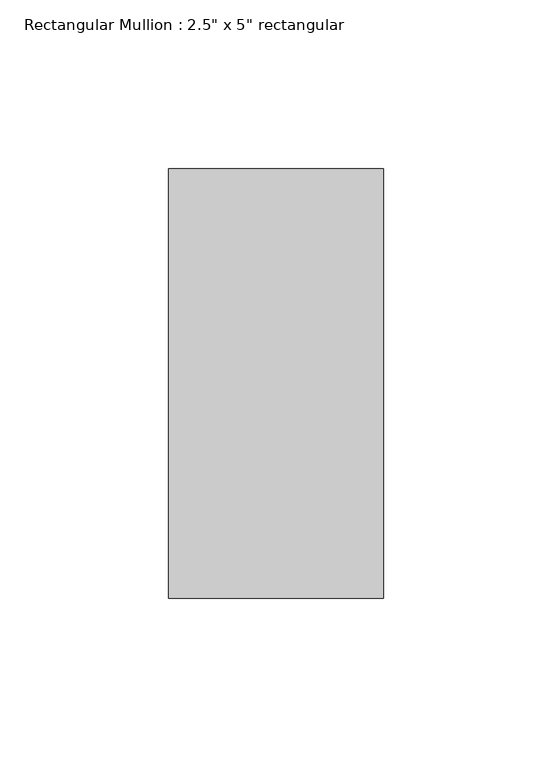
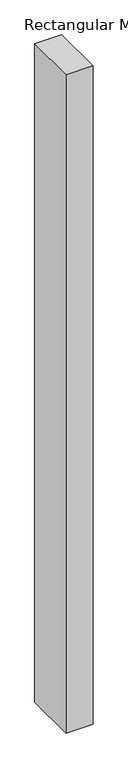
"""IFC4 building model written with IfcOpenShell, lengths in millimetres: member geometry."""

from ifc_helpers import new_model, si_unit, frame, origin, place, context, project, spatial, polyline, outline, extrude, source, transform, mapped, element, save


def member_e2524bce(model_context):
    return source(origin(), model_context, "Body", "SweptSolid", [
        extrude(outline(polyline([(0.0, 63.5), (0.0, -63.5), (-63.5, -63.5), (-63.5, 63.5), (0.0, 63.5)])), frame((0.0, 0.0, -1634.3549218), z_axis=(0.0, 0.0, 1.0), x_axis=(1.0, 0.0, 0.0)), (0.0, 0.0, 1.0), 1634.3549218),
    ])


if __name__ == "__main__":
    model = new_model("IFC4")
    model_context = context("Model", 3, world=origin())
    ifc_project = project(units=[si_unit("LENGTHUNIT", "METRE", prefix="MILLI")], contexts=[model_context])
    site = spatial("IfcSite", under=ifc_project)
    building = spatial("IfcBuilding", under=site)
    placement = place(None, origin())
    member_shape = member_e2524bce(model_context)
    element("IfcMember", 1, ObjectType="Rectangular Mullion : 2.5\" x 5\" rectangular", at=placement, inside=building, context=model_context, shape_type="MappedRepresentation", body=[
        mapped(member_shape, transform((0.0, 0.0, 0.0), x_axis=(1.0, 0.0, 0.0), y_axis=(0.0, 1.0, 0.0), z_axis=(0.0, 0.0, 1.0))),
    ])
    save(model, "model.ifc")

# Revit data of these elements
# Type "Rectangular Mullion : 2.5\" x 5\" rectangular"
#   built-in parameter 1007304 = 0.416667 (stored number, unit not read)
#   built-in parameter 1007301 = 0.104167 (stored number, unit not read)
#   built-in parameter 1007300 = 0.104167 (stored number, unit not read)
# Element 1 (IfcMember, "Rectangular Mullion : 2.5\" x 5\" rectangular")
#   Materials on its faces: "Aluminum"
# Materials
#   "Aluminum": class "Metal", colour RGB 247 247 247, transparency 0, Description = "Aluminum 6061", Cost = 0
